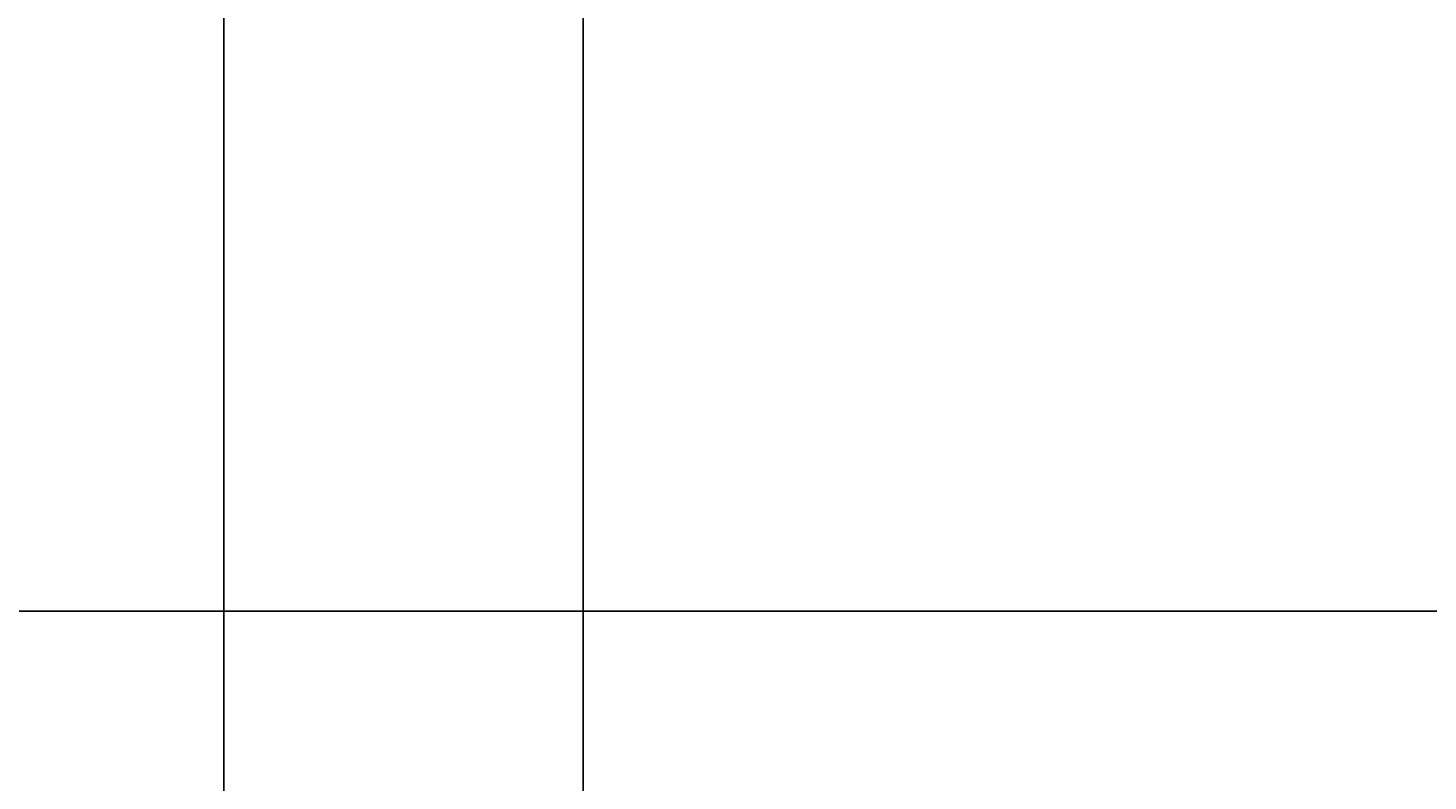
# Model space of a CAD drawing. Units: inches. Extents: x 35362 to 73946, y 43607 to 67532.
# Tile 17 of 134: x 47763 to 49302, y 45263 to 46091. Entities that reach past the tile are written whole.
import ezdxf

# ---------------------------------------------------------------- set-up
doc = ezdxf.new("R2010")
doc.units = ezdxf.units.IN
doc.header["$MEASUREMENT"] = 0
doc.layers.add('A-ANNO-DIMS', color=2, linetype='Continuous', lineweight=18)
doc.styles.get("Standard").update_dxf_attribs({"font": 'arial.ttf'})
doc.dimstyles.get("Standard").update_dxf_attribs({"dimtxt": 0.18, "dimasz": 0.18, "dimexe": 0.18, "dimexo": 0.0625, "dimgap": 0.09, "dimtad": 0, "dimtih": 1, "dimtoh": 1, "dimdec": 4, "dimzin": 0, "dimdsep": 46, "dimtxsty": 'Standard', "dimcen": 0.09, "dimadec": 0, "dimazin": 0, "dimtfac": 1, "dimtdec": 4, "dimtofl": 0, "dimtmove": 0, "dimatfit": 3, "dimfxl": 1, "dimtolj": 1, "dimtzin": 0, "dimarcsym": 0})

# ---------------------------------------------------------------- blocks, each defined once
blk = doc.blocks.new('*D5')
at = {"layer": 'A-ANNO-DIMS', "color": 0, "lineweight": -2, "transparency": 16777216}
for p, q in [((37121.9, 46919.3), (37121.9, 43606.7)), ((69871.5, 45449.8), (69871.5, 43606.7)), ((37122.1, 43606.9), (53496.3, 43606.9)), ((69871.3, 43606.9), (53497.2, 43606.9))]:
    blk.add_line(p, q, dxfattribs=at)
at = {"layer": 'A-ANNO-DIMS', "color": 0, "transparency": 16777216}
for points in [[(37122.1, 43606.9), (37122.1, 43606.8), (37121.9, 43606.9)], [(69871.3, 43606.9), (69871.3, 43606.8), (69871.5, 43606.9)]]:
    blk.add_solid(points, dxfattribs=at)
at = {"layer": 'Defpoints', "color": 0, "transparency": 16777216}
for p in [(37121.9, 46919.4), (69871.5, 45449.9), (69871.5, 43606.9)]:
    blk.add_point(p, dxfattribs=at)
at = {"layer": 'A-ANNO-DIMS', "color": 0, "transparency": 16777216, "insert": (53496.7, 43606.9), "char_height": 0.18, "attachment_point": 5}
blk.add_mtext('\\A1;32750', dxfattribs=at)
blk = doc.blocks.new('*D11')
at = {"layer": 'A-ANNO-DIMS', "color": 0, "lineweight": -2, "transparency": 16777216}
for p, q in [((47978.7, 56028.8), (47978.7, 43606.7)), ((53109.8, 56028.8), (53109.8, 43606.7)), ((47978.8, 43606.9), (50543.9, 43606.9)), ((53109.6, 43606.9), (50544.6, 43606.9))]:
    blk.add_line(p, q, dxfattribs=at)
at = {"layer": 'A-ANNO-DIMS', "color": 0, "transparency": 16777216}
for points in [[(47978.8, 43606.9), (47978.8, 43606.8), (47978.7, 43606.9)], [(53109.6, 43606.9), (53109.6, 43606.8), (53109.8, 43606.9)]]:
    blk.add_solid(points, dxfattribs=at)
at = {"layer": 'Defpoints', "color": 0, "transparency": 16777216}
for p in [(47978.7, 56028.8), (53109.8, 56028.8), (53109.8, 43606.9)]:
    blk.add_point(p, dxfattribs=at)
at = {"layer": 'A-ANNO-DIMS', "color": 0, "transparency": 16777216, "insert": (50544.2, 43606.9), "char_height": 0.18, "attachment_point": 5}
blk.add_mtext('\\A1;5131', dxfattribs=at)
blk = doc.blocks.new('*D13')
at = {"layer": 'A-ANNO-DIMS', "color": 0, "lineweight": -2, "transparency": 16777216}
for p, q in [((48373.5, 51694), (48373.5, 43606.7)), ((51029, 51694), (51029, 43606.7)), ((48373.7, 43606.9), (49700.8, 43606.9)), ((51028.9, 43606.9), (49701.7, 43606.9))]:
    blk.add_line(p, q, dxfattribs=at)
at = {"layer": 'A-ANNO-DIMS', "color": 0, "transparency": 16777216}
for points in [[(48373.7, 43606.9), (48373.7, 43606.8), (48373.5, 43606.9)], [(51028.9, 43606.9), (51028.9, 43606.8), (51029, 43606.9)]]:
    blk.add_solid(points, dxfattribs=at)
at = {"layer": 'Defpoints', "color": 0, "transparency": 16777216}
for p in [(48373.5, 51694.1), (51029, 51694.1), (51029, 43606.9)]:
    blk.add_point(p, dxfattribs=at)
at = {"layer": 'A-ANNO-DIMS', "color": 0, "transparency": 16777216, "insert": (49701.3, 43606.9), "char_height": 0.18, "attachment_point": 5}
blk.add_mtext('\\A1;2655.6', dxfattribs=at)
blk = doc.blocks.new('*D27')
at = {"layer": 'A-ANNO-DIMS', "color": 0, "lineweight": -2, "transparency": 16777216}
for p, q in [((47978.7, 56028.8), (47978.7, 43606.7)), ((48373.5, 53429), (48373.5, 43606.7)), ((47978.8, 43606.9), (48175.7, 43606.9)), ((48373.3, 43606.9), (48176.5, 43606.9))]:
    blk.add_line(p, q, dxfattribs=at)
at = {"layer": 'A-ANNO-DIMS', "color": 0, "transparency": 16777216}
for points in [[(47978.8, 43606.9), (47978.8, 43606.8), (47978.7, 43606.9)], [(48373.3, 43606.9), (48373.3, 43606.8), (48373.5, 43606.9)]]:
    blk.add_solid(points, dxfattribs=at)
at = {"layer": 'Defpoints', "color": 0, "transparency": 16777216}
for p in [(47978.7, 56028.8), (48373.5, 53429), (48373.5, 43606.9)]:
    blk.add_point(p, dxfattribs=at)
at = {"layer": 'A-ANNO-DIMS', "color": 0, "transparency": 16777216, "insert": (48176.1, 43606.9), "char_height": 0.18, "attachment_point": 5}
blk.add_mtext('\\A1;394.8', dxfattribs=at)
blk = doc.blocks.new('*D67')
at = {"layer": 'A-ANNO-DIMS', "color": 0, "lineweight": -2, "transparency": 16777216}
for p, q in [((56873.5, 53351.5), (35361.8, 53351.5)), ((35361.9, 53351.3), (35361.9, 49400.9)), ((35361.9, 45450.1), (35361.9, 49400.5)), ((53793.6, 45449.9), (35361.8, 45449.9))]:
    blk.add_line(p, q, dxfattribs=at)
at = {"layer": 'A-ANNO-DIMS', "color": 0, "transparency": 16777216}
for points in [[(35361.9, 53351.3), (35362, 53351.3), (35361.9, 53351.5)], [(35361.9, 45450.1), (35362, 45450.1), (35361.9, 45449.9)]]:
    blk.add_solid(points, dxfattribs=at)
at = {"layer": 'Defpoints', "color": 0, "transparency": 16777216}
for p in [(35361.9, 53351.5), (56873.6, 53351.5), (53793.6, 45449.9)]:
    blk.add_point(p, dxfattribs=at)
at = {"layer": 'A-ANNO-DIMS', "color": 0, "transparency": 16777216, "insert": (35361.9, 49400.7), "char_height": 0.18, "attachment_point": 5}
blk.add_mtext('\\A1;7901.6', dxfattribs=at)

msp = doc.modelspace()

# ---------------------------------------------------------------- dimensions: what is measured, and where the dimension line sits
at = {"layer": 'A-ANNO-DIMS'}
for base, p1, p2, override, picture, middle in [((53109.76, 43606.859), (47978.665, 56028.836), (53109.76, 56028.836), {"dimdec": 0, "dimlfac": 1, "dimrnd": 0, "dimzin": 0, "dimdsep": 46, "dimlunit": 2}, '*D11', (50544.212, 43606.859)), ((48373.492, 43606.859), (47978.665, 56028.836), (48373.492, 53429.019), {"dimdec": 1, "dimlfac": 1, "dimrnd": 0, "dimzin": 0, "dimdsep": 46, "dimlunit": 2}, '*D27', (48176.078, 43606.859)), ((51029.043, 43606.859), (48373.492, 51694.087), (51029.043, 51694.087), {"dimdec": 1, "dimlfac": 1, "dimrnd": 0, "dimzin": 0, "dimdsep": 46, "dimlunit": 2}, '*D13', (49701.267, 43606.859)), ((69871.496, 43606.859), (37121.949, 46919.381), (69871.496, 45449.894), {"dimdec": 0, "dimlfac": 1, "dimrnd": 0, "dimzin": 0, "dimdsep": 46, "dimlunit": 2}, '*D5', (53496.723, 43606.859))]:
    dim = msp.add_linear_dim(base=base, p1=p1, p2=p2, dimstyle='Standard', override=override, dxfattribs=at)
    dim.commit()
    dim.dimension.update_dxf_attribs({"geometry": picture, "text_midpoint": middle})
dim = msp.add_linear_dim(base=(35361.949, 53351.529), p1=(53793.638, 45449.894), p2=(56873.602, 53351.529), angle=90, dimstyle='Standard', override={"dimdec": 1, "dimlfac": 1, "dimrnd": 0, "dimzin": 0, "dimdsep": 46, "dimlunit": 2}, dxfattribs=at)
dim.commit()
dim.dimension.update_dxf_attribs({"geometry": '*D67', "text_midpoint": (35361.949, 49400.712)})

doc.saveas('drawing.dxf')
